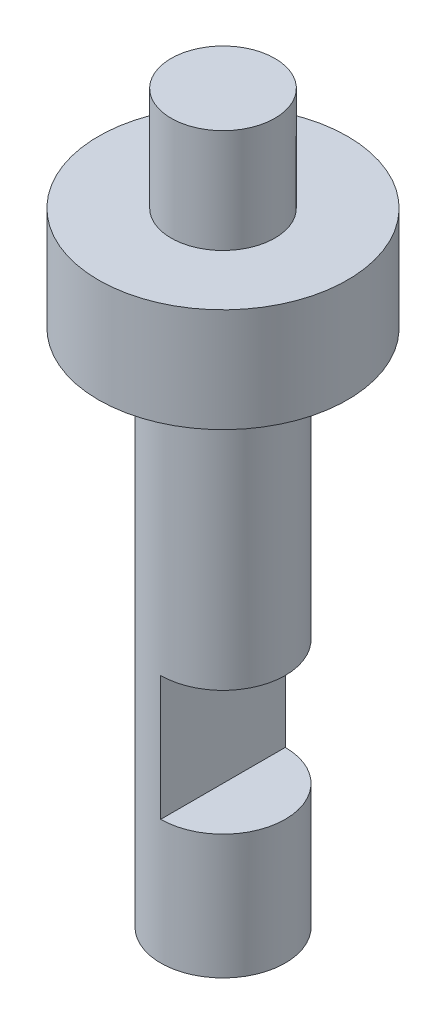
ISO-10303-21;
HEADER;
FILE_DESCRIPTION(('STEP AP214'),'2;1');
FILE_NAME('part.step','',(''),(''),'','','');
FILE_SCHEMA(('AUTOMOTIVE_DESIGN { 1 0 10303 214 1 1 1 1 }'));
ENDSEC;
DATA;
#1=APPLICATION_CONTEXT('core data for automotive mechanical design processes');
#2=APPLICATION_PROTOCOL_DEFINITION('international standard','automotive_design',2000,#1);
#3=PRODUCT_CONTEXT('',#1,'mechanical');
#4=PRODUCT('Part','Part','',(#3));
#5=PRODUCT_RELATED_PRODUCT_CATEGORY('part','',(#4));
#6=PRODUCT_DEFINITION_FORMATION('','',#4);
#7=PRODUCT_DEFINITION_CONTEXT('part definition',#1,'design');
#8=PRODUCT_DEFINITION('design','',#6,#7);
#9=PRODUCT_DEFINITION_SHAPE('','',#8);
#10=(LENGTH_UNIT() NAMED_UNIT(*) SI_UNIT(.MILLI.,.METRE.));
#11=(NAMED_UNIT(*) PLANE_ANGLE_UNIT() SI_UNIT($,.RADIAN.));
#12=(NAMED_UNIT(*) SI_UNIT($,.STERADIAN.) SOLID_ANGLE_UNIT());
#13=UNCERTAINTY_MEASURE_WITH_UNIT(LENGTH_MEASURE(1.E-05),#10,'distance_accuracy_value','');
#14=(GEOMETRIC_REPRESENTATION_CONTEXT(3) GLOBAL_UNCERTAINTY_ASSIGNED_CONTEXT((#13)) GLOBAL_UNIT_ASSIGNED_CONTEXT((#10,
#11,#12)) REPRESENTATION_CONTEXT('',''));
#15=CARTESIAN_POINT('',(0.,0.,0.));
#16=DIRECTION('',(0.,0.,1.));
#17=DIRECTION('',(1.,0.,0.));
#18=AXIS2_PLACEMENT_3D('',#15,#16,#17);
#19=CARTESIAN_POINT('',(0.,0.,0.));
#20=DIRECTION('',(0.,-1.,0.));
#21=DIRECTION('',(0.,0.,-1.));
#22=AXIS2_PLACEMENT_3D('',#19,#20,#21);
#23=PLANE('',#22);
#24=CARTESIAN_POINT('',(0.,0.,0.));
#25=DIRECTION('',(0.,-1.,0.));
#26=DIRECTION('',(0.,0.,-1.));
#27=AXIS2_PLACEMENT_3D('',#24,#25,#26);
#28=CIRCLE('',#27,2.5);
#29=CARTESIAN_POINT('',(0.,0.,-2.5));
#30=VERTEX_POINT('',#29);
#31=EDGE_CURVE('E67',#30,#30,#28,.T.);
#32=ORIENTED_EDGE('',*,*,#31,.F.);
#33=EDGE_LOOP('',(#32));
#34=FACE_BOUND('',#33,.T.);
#35=ADVANCED_FACE('F39',(#34),#23,.F.);
#36=CARTESIAN_POINT('',(0.,-35.,0.));
#37=DIRECTION('',(0.,-1.,0.));
#38=DIRECTION('',(0.,0.,-1.));
#39=AXIS2_PLACEMENT_3D('',#36,#37,#38);
#40=CYLINDRICAL_SURFACE('',#39,2.5);
#41=CARTESIAN_POINT('',(0.,-5.,0.));
#42=DIRECTION('',(0.,-1.,0.));
#43=DIRECTION('',(0.,0.,-1.));
#44=AXIS2_PLACEMENT_3D('',#41,#42,#43);
#45=CIRCLE('',#44,2.5);
#46=CARTESIAN_POINT('',(0.,-5.,-2.5));
#47=VERTEX_POINT('',#46);
#48=EDGE_CURVE('E81',#47,#47,#45,.T.);
#49=ORIENTED_EDGE('',*,*,#48,.F.);
#50=EDGE_LOOP('',(#49));
#51=FACE_BOUND('',#50,.T.);
#52=ORIENTED_EDGE('',*,*,#31,.T.);
#53=EDGE_LOOP('',(#52));
#54=FACE_BOUND('',#53,.T.);
#55=ADVANCED_FACE('F107',(#51,#54),#40,.T.);
#56=CARTESIAN_POINT('',(-2.5,-5.,0.));
#57=DIRECTION('',(0.,-1.,0.));
#58=DIRECTION('',(0.,0.,-1.));
#59=AXIS2_PLACEMENT_3D('',#56,#57,#58);
#60=PLANE('',#59);
#61=CARTESIAN_POINT('',(0.,-5.,0.));
#62=DIRECTION('',(0.,-1.,0.));
#63=DIRECTION('',(0.,0.,-1.));
#64=AXIS2_PLACEMENT_3D('',#61,#62,#63);
#65=CIRCLE('',#64,6.);
#66=CARTESIAN_POINT('',(0.,-5.,-6.));
#67=VERTEX_POINT('',#66);
#68=EDGE_CURVE('E82',#67,#67,#65,.T.);
#69=ORIENTED_EDGE('',*,*,#68,.F.);
#70=EDGE_LOOP('',(#69));
#71=FACE_BOUND('',#70,.T.);
#72=ORIENTED_EDGE('',*,*,#48,.T.);
#73=EDGE_LOOP('',(#72));
#74=FACE_BOUND('',#73,.T.);
#75=ADVANCED_FACE('F114',(#71,#74),#60,.F.);
#76=CARTESIAN_POINT('',(0.,-35.,0.));
#77=DIRECTION('',(0.,-1.,0.));
#78=DIRECTION('',(0.,0.,-1.));
#79=AXIS2_PLACEMENT_3D('',#76,#77,#78);
#80=CYLINDRICAL_SURFACE('',#79,6.);
#81=CARTESIAN_POINT('',(0.,-10.,0.));
#82=DIRECTION('',(0.,-1.,0.));
#83=DIRECTION('',(0.,0.,-1.));
#84=AXIS2_PLACEMENT_3D('',#81,#82,#83);
#85=CIRCLE('',#84,6.);
#86=CARTESIAN_POINT('',(0.,-10.,-6.));
#87=VERTEX_POINT('',#86);
#88=EDGE_CURVE('E86',#87,#87,#85,.T.);
#89=ORIENTED_EDGE('',*,*,#88,.F.);
#90=EDGE_LOOP('',(#89));
#91=FACE_BOUND('',#90,.T.);
#92=ORIENTED_EDGE('',*,*,#68,.T.);
#93=EDGE_LOOP('',(#92));
#94=FACE_BOUND('',#93,.T.);
#95=ADVANCED_FACE('F119',(#91,#94),#80,.T.);
#96=CARTESIAN_POINT('',(-6.,-10.,0.));
#97=DIRECTION('',(0.,1.,0.));
#98=DIRECTION('',(0.,0.,1.));
#99=AXIS2_PLACEMENT_3D('',#96,#97,#98);
#100=PLANE('',#99);
#101=CARTESIAN_POINT('',(0.,-10.,0.));
#102=DIRECTION('',(0.,-1.,0.));
#103=DIRECTION('',(0.,0.,-1.));
#104=AXIS2_PLACEMENT_3D('',#101,#102,#103);
#105=CIRCLE('',#104,3.);
#106=CARTESIAN_POINT('',(0.,-10.,-3.));
#107=VERTEX_POINT('',#106);
#108=EDGE_CURVE('E93',#107,#107,#105,.T.);
#109=ORIENTED_EDGE('',*,*,#108,.F.);
#110=EDGE_LOOP('',(#109));
#111=FACE_BOUND('',#110,.T.);
#112=ORIENTED_EDGE('',*,*,#88,.T.);
#113=EDGE_LOOP('',(#112));
#114=FACE_BOUND('',#113,.T.);
#115=ADVANCED_FACE('F130',(#111,#114),#100,.F.);
#116=CARTESIAN_POINT('',(0.,-35.,0.));
#117=DIRECTION('',(0.,-1.,0.));
#118=DIRECTION('',(0.,0.,-1.));
#119=AXIS2_PLACEMENT_3D('',#116,#117,#118);
#120=CYLINDRICAL_SURFACE('',#119,3.);
#121=DIRECTION('',(0.,-1.,0.));
#122=VECTOR('',#121,1.);
#123=CARTESIAN_POINT('',(0.,-35.,3.));
#124=LINE('',#123,#122);
#125=CARTESIAN_POINT('',(0.,-29.,3.));
#126=VERTEX_POINT('',#125);
#127=CARTESIAN_POINT('',(0.,-23.,3.));
#128=VERTEX_POINT('',#127);
#129=EDGE_CURVE('E68',#126,#128,#124,.F.);
#130=ORIENTED_EDGE('',*,*,#129,.T.);
#131=CARTESIAN_POINT('',(0.,-23.,0.));
#132=DIRECTION('',(0.,1.,0.));
#133=DIRECTION('',(0.,0.,1.));
#134=AXIS2_PLACEMENT_3D('',#131,#132,#133);
#135=CIRCLE('',#134,3.);
#136=CARTESIAN_POINT('',(0.,-23.,-3.));
#137=VERTEX_POINT('',#136);
#138=EDGE_CURVE('E11',#128,#137,#135,.T.);
#139=ORIENTED_EDGE('',*,*,#138,.T.);
#140=DIRECTION('',(0.,-1.,0.));
#141=VECTOR('',#140,1.);
#142=CARTESIAN_POINT('',(0.,-35.,-3.));
#143=LINE('',#142,#141);
#144=CARTESIAN_POINT('',(0.,-29.,-3.));
#145=VERTEX_POINT('',#144);
#146=EDGE_CURVE('E46',#137,#145,#143,.T.);
#147=ORIENTED_EDGE('',*,*,#146,.T.);
#148=CARTESIAN_POINT('',(0.,-29.,0.));
#149=DIRECTION('',(0.,-1.,0.));
#150=DIRECTION('',(0.,0.,-1.));
#151=AXIS2_PLACEMENT_3D('',#148,#149,#150);
#152=CIRCLE('',#151,3.);
#153=EDGE_CURVE('E63',#145,#126,#152,.T.);
#154=ORIENTED_EDGE('',*,*,#153,.T.);
#155=EDGE_LOOP('',(#130,#139,#147,#154));
#156=FACE_BOUND('',#155,.T.);
#157=CARTESIAN_POINT('',(0.,-35.,0.));
#158=DIRECTION('',(0.,-1.,0.));
#159=DIRECTION('',(0.,0.,-1.));
#160=AXIS2_PLACEMENT_3D('',#157,#158,#159);
#161=CIRCLE('',#160,3.);
#162=CARTESIAN_POINT('',(0.,-35.,-3.));
#163=VERTEX_POINT('',#162);
#164=EDGE_CURVE('E94',#163,#163,#161,.T.);
#165=ORIENTED_EDGE('',*,*,#164,.F.);
#166=EDGE_LOOP('',(#165));
#167=FACE_BOUND('',#166,.T.);
#168=ORIENTED_EDGE('',*,*,#108,.T.);
#169=EDGE_LOOP('',(#168));
#170=FACE_BOUND('',#169,.T.);
#171=ADVANCED_FACE('F76',(#156,#167,#170),#120,.T.);
#172=CARTESIAN_POINT('',(-3.,-35.,0.));
#173=DIRECTION('',(0.,1.,0.));
#174=DIRECTION('',(0.,0.,1.));
#175=AXIS2_PLACEMENT_3D('',#172,#173,#174);
#176=PLANE('',#175);
#177=ORIENTED_EDGE('',*,*,#164,.T.);
#178=EDGE_LOOP('',(#177));
#179=FACE_BOUND('',#178,.T.);
#180=ADVANCED_FACE('F104',(#179),#176,.F.);
#181=CARTESIAN_POINT('',(0.,-23.,-9.5));
#182=DIRECTION('',(-1.,0.,0.));
#183=DIRECTION('',(0.,-1.,0.));
#184=AXIS2_PLACEMENT_3D('',#181,#182,#183);
#185=PLANE('',#184);
#186=DIRECTION('',(0.,0.,1.));
#187=VECTOR('',#186,1.);
#188=CARTESIAN_POINT('',(0.,-23.,-9.5));
#189=LINE('',#188,#187);
#190=EDGE_CURVE('E74',#137,#128,#189,.T.);
#191=ORIENTED_EDGE('',*,*,#190,.T.);
#192=ORIENTED_EDGE('',*,*,#129,.F.);
#193=DIRECTION('',(0.,0.,1.));
#194=VECTOR('',#193,1.);
#195=CARTESIAN_POINT('',(0.,-29.,-9.5));
#196=LINE('',#195,#194);
#197=EDGE_CURVE('E55',#145,#126,#196,.T.);
#198=ORIENTED_EDGE('',*,*,#197,.F.);
#199=ORIENTED_EDGE('',*,*,#146,.F.);
#200=EDGE_LOOP('',(#191,#192,#198,#199));
#201=FACE_BOUND('',#200,.T.);
#202=ADVANCED_FACE('F71',(#201),#185,.F.);
#203=CARTESIAN_POINT('',(0.,-23.,-9.5));
#204=DIRECTION('',(0.,1.,0.));
#205=DIRECTION('',(0.,0.,1.));
#206=AXIS2_PLACEMENT_3D('',#203,#204,#205);
#207=PLANE('',#206);
#208=ORIENTED_EDGE('',*,*,#190,.F.);
#209=ORIENTED_EDGE('',*,*,#138,.F.);
#210=EDGE_LOOP('',(#208,#209));
#211=FACE_BOUND('',#210,.T.);
#212=ADVANCED_FACE('F100',(#211),#207,.F.);
#213=CARTESIAN_POINT('',(0.,-29.,-9.5));
#214=DIRECTION('',(0.,-1.,0.));
#215=DIRECTION('',(0.,0.,-1.));
#216=AXIS2_PLACEMENT_3D('',#213,#214,#215);
#217=PLANE('',#216);
#218=ORIENTED_EDGE('',*,*,#197,.T.);
#219=ORIENTED_EDGE('',*,*,#153,.F.);
#220=EDGE_LOOP('',(#218,#219));
#221=FACE_BOUND('',#220,.T.);
#222=ADVANCED_FACE('F64',(#221),#217,.F.);
#223=CLOSED_SHELL('',(#35,#55,#75,#95,#115,#171,#180,#202,#212,#222));
#224=MANIFOLD_SOLID_BREP('B2',#223);
#225=ADVANCED_BREP_SHAPE_REPRESENTATION('',(#18,#224),#14);
#226=SHAPE_DEFINITION_REPRESENTATION(#9,#225);
ENDSEC;
END-ISO-10303-21;
